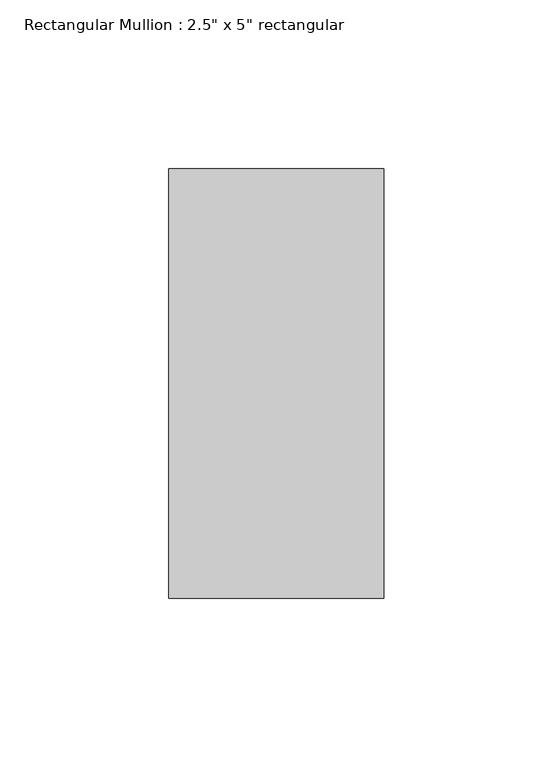
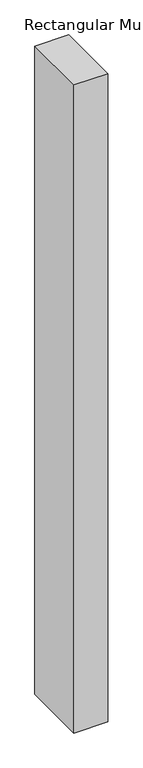
"""IFC4 building model written with IfcOpenShell, lengths in millimetres: member geometry."""

from ifc_helpers import new_model, si_unit, frame, origin, place, context, project, spatial, polyline, outline, extrude, source, transform, mapped, element, save


def member_798c2a08(model_context):
    return source(origin(), model_context, "Body", "SweptSolid", [
        extrude(outline(polyline([(0.0, 63.5), (0.0, -63.5), (-63.5, -63.5), (-63.5, 63.5), (0.0, 63.5)])), frame((0.0, 0.0, -1289.05), z_axis=(0.0, 0.0, 1.0), x_axis=(1.0, 0.0, 0.0)), (0.0, 0.0, 1.0), 1289.05),
    ])


if __name__ == "__main__":
    model = new_model("IFC4")
    model_context = context("Model", 3, world=origin())
    ifc_project = project(units=[si_unit("LENGTHUNIT", "METRE", prefix="MILLI")], contexts=[model_context])
    site = spatial("IfcSite", under=ifc_project)
    building = spatial("IfcBuilding", under=site)
    placement = place(None, origin())
    member_shape = member_798c2a08(model_context)
    element("IfcMember", 1, ObjectType="Rectangular Mullion : 2.5\" x 5\" rectangular", at=placement, inside=building, context=model_context, shape_type="MappedRepresentation", body=[
        mapped(member_shape, transform((0.0, 0.0, 0.0), x_axis=(1.0, 0.0, 0.0), y_axis=(0.0, 1.0, 0.0), z_axis=(0.0, 0.0, 1.0))),
    ])
    save(model, "model.ifc")

# Revit data of these elements
# Type "Rectangular Mullion : 2.5\" x 5\" rectangular"
#   built-in parameter 1007304 = 0.416667 (stored number, unit not read)
#   built-in parameter 1007301 = 0.104167 (stored number, unit not read)
#   built-in parameter 1007300 = 0.104167 (stored number, unit not read)
# Element 1 (IfcMember, "Rectangular Mullion : 2.5\" x 5\" rectangular")
#   Materials on its faces: "Aluminum"
# Materials
#   "Aluminum": class "Metal", colour RGB 247 247 247, transparency 0, Description = "Aluminum 6061", Cost = 0
